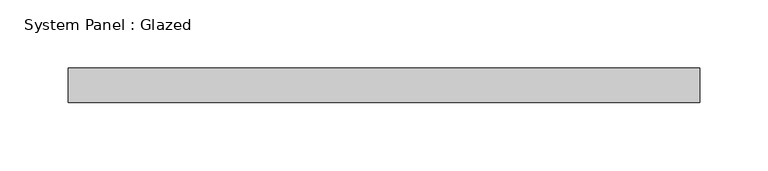
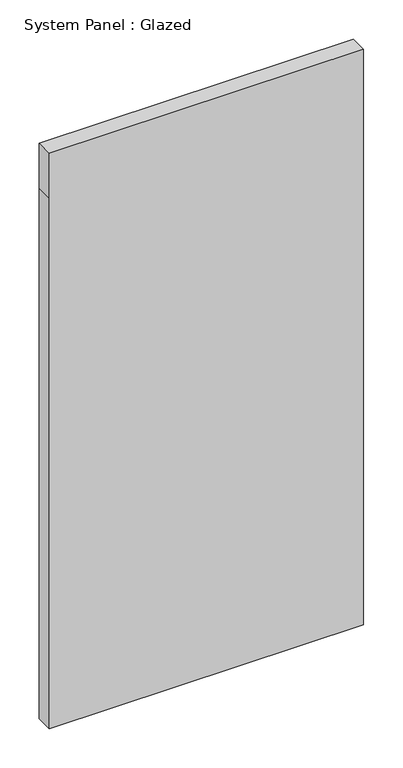
"""IFC4 building model written with IfcOpenShell, lengths in millimetres: plate geometry, System Panel : Glazed."""

from ifc_helpers import new_model, si_unit, frame, origin, place, context, project, spatial, polyline, outline, extrude, source, transform, mapped, element, save


def system_panel_glazed_40386fdd(model_context):
    return source(origin(), model_context, "Body", "SweptSolid", [
        extrude(outline(polyline([(0.0, -231.775), (0.0, 231.775), (826.3127727, 231.775), (896.1627727, 231.775), (896.1627727, -231.775), (826.3127727, -231.775), (0.0, -231.775)])), frame((0.0, 19.05, 0.0), z_axis=(0.0, 1.0, 0.0), x_axis=(0.0, 0.0, 1.0)), (0.0, 0.0, 1.0), 25.4),
    ])


if __name__ == "__main__":
    model = new_model("IFC4")
    model_context = context("Model", 3, world=origin())
    ifc_project = project(units=[si_unit("LENGTHUNIT", "METRE", prefix="MILLI")], contexts=[model_context])
    site = spatial("IfcSite", under=ifc_project)
    building = spatial("IfcBuilding", under=site)
    placement = place(None, origin())
    system_panel_glazed_shape = system_panel_glazed_40386fdd(model_context)
    element("IfcPlate", 1, ObjectType="System Panel : Glazed", at=placement, inside=building, context=model_context, shape_type="MappedRepresentation", body=[
        mapped(system_panel_glazed_shape, transform((0.0, 0.0, 0.0), x_axis=(1.0, 0.0, 0.0), y_axis=(0.0, 1.0, 0.0), z_axis=(0.0, 0.0, 1.0))),
    ])
    save(model, "model.ifc")

# Revit data of these elements
# Type "System Panel : Glazed"
#   Construction Type Id = "GSP4R"
#   Analytic Construction = "1/8 in Pilkington single glazing"
#   Visual Light Transmittance = 0.9
#   Solar Heat Gain Coefficient = 0.86
#   Heat Transfer Coefficient (U) = 1.18115 BTU/(h·ft²·°F)
#   Define Thermal Properties by = 1
# Element 1 (IfcPlate, "System Panel : Glazed")
#   Materials on its faces: "Glass"
# Materials
#   "Glass": class "Glass", colour RGB 0 128 192, transparency 0.75, Description = "Soda Lime Glass", Cost = 0
